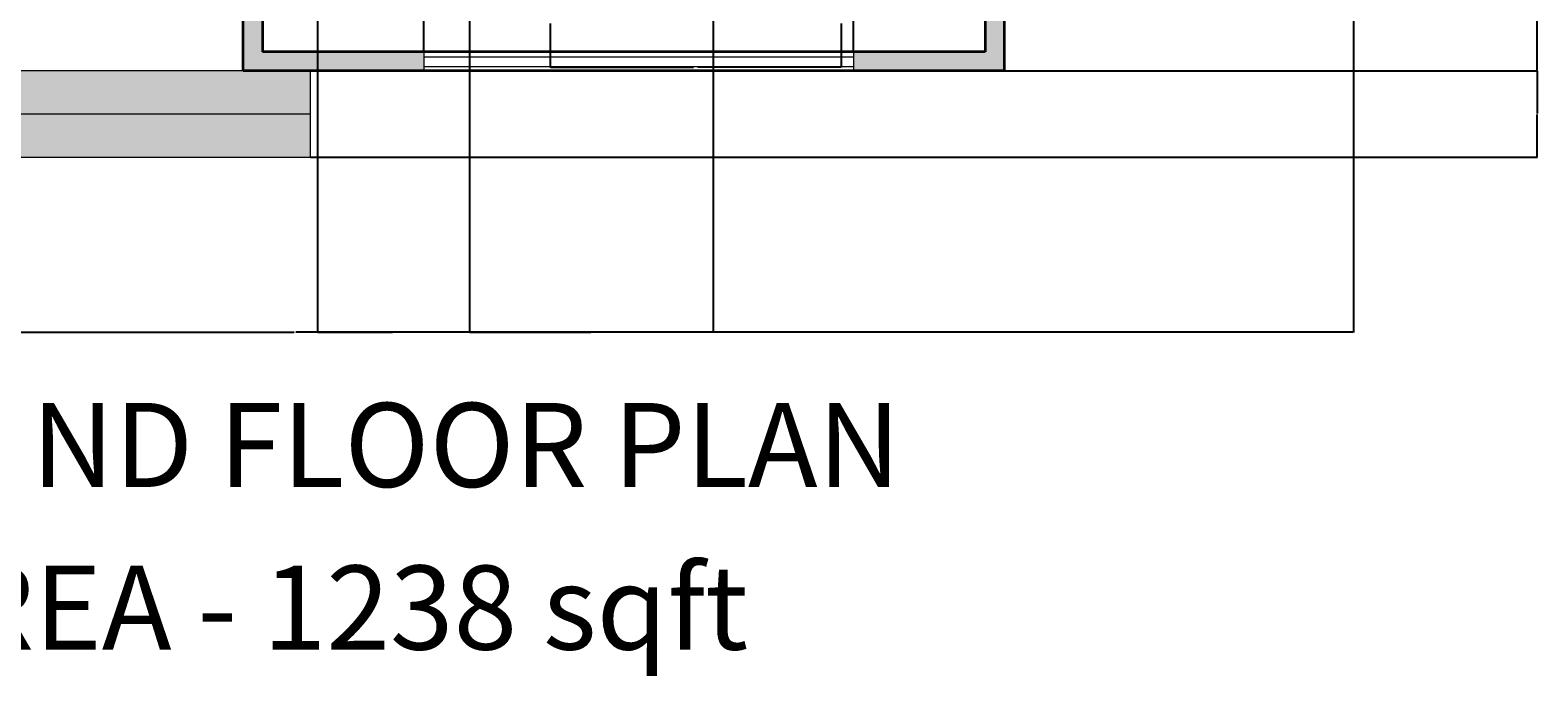
# Model space of a CAD drawing. Units: inches. Extents: x 192 to 1361, y -1362 to 367.
# Tile 10 of 23: x 649 to 1361, y -1362 to -1057. Entities that reach past the tile are written whole.
import ezdxf

# ---------------------------------------------------------------- set-up
doc = ezdxf.new("R2010")
doc.units = ezdxf.units.IN
doc.header["$MEASUREMENT"] = 0
for name, color, linetype, lineweight in [('A-ANNO-DIMS', 2, 'Continuous', 18), ('A-ANNO-TITL', 7, 'Continuous', 35), ('A-FLOR', 8, 'Continuous', 18), ('A-FLOR-STRS', 7, 'Continuous', 18), ('A-WALL-PATT', 250, 'Continuous', 13), ('walls', 7, 'Continuous', 35), ('windows', 4, 'Continuous', 18)]:
    doc.layers.add(name, color=color, linetype=linetype, lineweight=lineweight)
doc.layers.add('A-FLOR-STRS-PATT', color=252, linetype='Continuous', lineweight=13, true_color=0x939598)
doc.styles.get("Standard").update_dxf_attribs({"font": 'arial.ttf'})
doc.dimstyles.get("Standard").update_dxf_attribs({"dimtxt": 0.18, "dimasz": 0.18, "dimexe": 0.18, "dimexo": 0.0625, "dimgap": 0.09, "dimtad": 0, "dimtih": 1, "dimtoh": 1, "dimzin": 0, "dimdsep": 46, "dimlunit": 3, "dimtxsty": 'Standard', "dimcen": 0.09, "dimadec": 0, "dimazin": 0, "dimtfac": 1, "dimtofl": 0, "dimtmove": 0, "dimatfit": 3, "dimfxl": 1, "dimtolj": 1, "dimtzin": 0, "dimarcsym": 0})

# ---------------------------------------------------------------- blocks, each defined once
blk = doc.blocks.new('*D27')
at = {"layer": 'A-ANNO-DIMS', "color": 0, "lineweight": -2, "transparency": 16777216}
for p, q in [((894.63, -1054.34), (894.63, -1075.05)), ((1031.96, -1054.34), (1031.96, -1075.05)), ((894.81, -1074.87), (962.32, -1074.87)), ((1031.78, -1074.87), (964.27, -1074.87))]:
    blk.add_line(p, q, dxfattribs=at)
at = {"layer": 'A-ANNO-DIMS', "color": 0, "transparency": 16777216}
for points in [[(894.81, -1074.84), (894.81, -1074.9), (894.63, -1074.87)], [(1031.78, -1074.84), (1031.78, -1074.9), (1031.96, -1074.87)]]:
    blk.add_solid(points, dxfattribs=at)
at = {"layer": 'Defpoints', "color": 0, "transparency": 16777216}
for p in [(894.63, -1054.27), (1031.96, -1054.27), (1031.96, -1074.87)]:
    blk.add_point(p, dxfattribs=at)
at = {"layer": 'A-ANNO-DIMS', "color": 0, "transparency": 16777216, "insert": (963.29, -1074.87), "char_height": 0.18, "attachment_point": 5}
blk.add_mtext('\\A1;SOFA 137 TYP.', dxfattribs=at)
blk = doc.blocks.new('*D47')
at = {"layer": 'A-ANNO-DIMS', "color": 0, "lineweight": -2, "transparency": 16777216}
for p, q in [((1273.57, -782.95), (1273.57, -1200.05)), ((274.89, -914.5), (274.89, -1200.05)), ((275.07, -1199.87), (773.84, -1199.87)), ((1273.39, -1199.87), (774.62, -1199.87))]:
    blk.add_line(p, q, dxfattribs=at)
at = {"layer": 'A-ANNO-DIMS', "color": 0, "transparency": 16777216}
for points in [[(275.07, -1199.84), (275.07, -1199.9), (274.89, -1199.87)], [(1273.39, -1199.84), (1273.39, -1199.9), (1273.57, -1199.87)]]:
    blk.add_solid(points, dxfattribs=at)
at = {"layer": 'Defpoints', "color": 0, "transparency": 16777216}
for p in [(1273.57, -782.89), (274.89, -914.44), (1273.57, -1199.87)]:
    blk.add_point(p, dxfattribs=at)
at = {"layer": 'A-ANNO-DIMS', "color": 0, "transparency": 16777216, "insert": (774.23, -1199.87), "char_height": 0.18, "attachment_point": 5}
blk.add_mtext('\\A1;998.7', dxfattribs=at)
blk = doc.blocks.new('*D59')
at = {"layer": 'A-ANNO-DIMS', "color": 0, "lineweight": -2, "transparency": 16777216}
for p, q in [((1273.63, -782.89), (1360.41, -782.89)), ((1360.23, -783.07), (1360.23, -929.58)), ((1360.23, -1076.44), (1360.23, -929.94)), ((1108.9, -1076.62), (1360.41, -1076.62))]:
    blk.add_line(p, q, dxfattribs=at)
at = {"layer": 'A-ANNO-DIMS', "color": 0, "transparency": 16777216}
for points in [[(1360.2, -783.07), (1360.26, -783.07), (1360.23, -782.89)], [(1360.2, -1076.44), (1360.26, -1076.44), (1360.23, -1076.62)]]:
    blk.add_solid(points, dxfattribs=at)
at = {"layer": 'Defpoints', "color": 0, "transparency": 16777216}
for p in [(1273.57, -782.89), (1360.23, -782.89), (1108.84, -1076.62)]:
    blk.add_point(p, dxfattribs=at)
at = {"layer": 'A-ANNO-DIMS', "color": 0, "transparency": 16777216, "insert": (1360.23, -929.76), "char_height": 0.18, "attachment_point": 5}
blk.add_mtext('\\A1;293.73', dxfattribs=at)
blk = doc.blocks.new('*D60')
at = {"layer": 'A-ANNO-DIMS', "color": 0, "lineweight": -2, "transparency": 16777216}
for p, q in [((1108.9, -1076.62), (1360.41, -1076.62)), ((1360.23, -1076.8), (1360.23, -1096.79)), ((1360.23, -1117.14), (1360.23, -1097.16)), ((781.62, -1117.32), (1360.41, -1117.32))]:
    blk.add_line(p, q, dxfattribs=at)
at = {"layer": 'A-ANNO-DIMS', "color": 0, "transparency": 16777216}
for points in [[(1360.2, -1076.8), (1360.26, -1076.8), (1360.23, -1076.62)], [(1360.2, -1117.14), (1360.26, -1117.14), (1360.23, -1117.32)]]:
    blk.add_solid(points, dxfattribs=at)
at = {"layer": 'Defpoints', "color": 0, "transparency": 16777216}
for p in [(1108.84, -1076.62), (781.55, -1117.32), (1360.23, -1117.32)]:
    blk.add_point(p, dxfattribs=at)
at = {"layer": 'A-ANNO-DIMS', "color": 0, "transparency": 16777216, "insert": (1360.23, -1096.97), "char_height": 0.18, "attachment_point": 5}
blk.add_mtext('\\A1;40.7', dxfattribs=at)
blk = doc.blocks.new('*D67')
at = {"layer": 'A-ANNO-DIMS', "color": 0, "lineweight": -2, "transparency": 16777216}
for p, q in [((784.8, -597.56), (784.8, -1200.05)), ((856.57, -597.56), (856.57, -1200.05)), ((784.98, -1199.87), (820.29, -1199.87)), ((856.39, -1199.87), (821.08, -1199.87))]:
    blk.add_line(p, q, dxfattribs=at)
at = {"layer": 'A-ANNO-DIMS', "color": 0, "transparency": 16777216}
for points in [[(784.98, -1199.84), (784.98, -1199.9), (784.8, -1199.87)], [(856.39, -1199.84), (856.39, -1199.9), (856.57, -1199.87)]]:
    blk.add_solid(points, dxfattribs=at)
at = {"layer": 'Defpoints', "color": 0, "transparency": 16777216}
for p in [(784.8, -597.5), (856.57, -597.5), (856.57, -1199.87)]:
    blk.add_point(p, dxfattribs=at)
at = {"layer": 'A-ANNO-DIMS', "color": 0, "transparency": 16777216, "insert": (820.69, -1199.87), "char_height": 0.18, "attachment_point": 5}
blk.add_mtext('\\A1;71.76', dxfattribs=at)
blk = doc.blocks.new('*D68')
at = {"layer": 'A-ANNO-DIMS', "color": 0, "lineweight": -2, "transparency": 16777216}
for p, q in [((856.57, -597.56), (856.57, -1200.05)), ((971.58, -597.56), (971.58, -1200.05)), ((856.75, -1199.87), (913.79, -1199.87)), ((971.4, -1199.87), (914.36, -1199.87))]:
    blk.add_line(p, q, dxfattribs=at)
at = {"layer": 'A-ANNO-DIMS', "color": 0, "transparency": 16777216}
for points in [[(856.75, -1199.84), (856.75, -1199.9), (856.57, -1199.87)], [(971.4, -1199.84), (971.4, -1199.9), (971.58, -1199.87)]]:
    blk.add_solid(points, dxfattribs=at)
at = {"layer": 'Defpoints', "color": 0, "transparency": 16777216}
for p in [(856.57, -597.5), (971.58, -597.5), (971.58, -1199.87)]:
    blk.add_point(p, dxfattribs=at)
at = {"layer": 'A-ANNO-DIMS', "color": 0, "transparency": 16777216, "insert": (914.07, -1199.87), "char_height": 0.18, "attachment_point": 5}
blk.add_mtext('\\A1;115', dxfattribs=at)
blk = doc.blocks.new('*D72')
at = {"layer": 'A-ANNO-DIMS', "color": 0, "lineweight": -2, "transparency": 16777216}
for p, q in [((835.08, -1067.56), (835.08, 367.39)), ((835.26, 367.21), (935.95, 367.21)), ((1037.58, 367.21), (936.88, 367.21)), ((1037.76, -1067.56), (1037.76, 367.39))]:
    blk.add_line(p, q, dxfattribs=at)
at = {"layer": 'A-ANNO-DIMS', "color": 0, "transparency": 16777216}
for points in [[(835.26, 367.24), (835.26, 367.18), (835.08, 367.21)], [(1037.58, 367.24), (1037.58, 367.18), (1037.76, 367.21)]]:
    blk.add_solid(points, dxfattribs=at)
at = {"layer": 'Defpoints', "color": 0, "transparency": 16777216}
for p in [(1037.76, 367.21), (835.08, -1067.62), (1037.76, -1067.62)]:
    blk.add_point(p, dxfattribs=at)
at = {"layer": 'A-ANNO-DIMS', "color": 0, "transparency": 16777216, "insert": (936.42, 367.21), "char_height": 0.18, "attachment_point": 5}
blk.add_mtext('\\A1;202.68', dxfattribs=at)

msp = doc.modelspace()

# ---------------------------------------------------------------- hatches: boundary and pattern name
at = {"layer": 'A-FLOR-STRS-PATT'}
h = msp.add_hatch(color=256, dxfattribs=at)
h.dxf.hatch_style = 1
h.paths.add_polyline_path([(781.5537, -1096.9736), (395.2768, -1096.9736), (395.2768, -1117.3227), (781.5537, -1117.3227)])
h.paths.add_polyline_path([(781.5537, -1076.6246), (749.8458, -1076.6246), (441.307, -1076.6246), (395.2768, -1076.6246), (395.2768, -1096.9736), (781.5537, -1096.9736)])
at = {"layer": 'A-WALL-PATT'}
h = msp.add_hatch(color=256, dxfattribs=at)
h.dxf.hatch_style = 1
h.paths.add_polyline_path([(309.5452, 191.102), (300.5452, 191.102), (300.5452, -126.898), (309.5452, -126.898), (309.5452, -117.898)])
h.paths.add_polyline_path([(420.798, 191.102), (337.3229, 191.102), (337.3229, 182.102), (420.798, 182.102)])
h.paths.add_polyline_path([(518.5452, 182.102), (625.4022, 182.102), (625.4022, 191.102), (509.5452, 191.102), (509.5452, 114.3262), (518.5452, 114.3262)])
h.paths.add_polyline_path([(842.5452, 191.102), (763.4438, 191.102), (763.4438, 182.102), (833.5452, 182.102), (833.5452, 161.1615), (836.8088, 161.1615), (842.5452, 161.1615)])
h.paths.add_polyline_path([(842.5452, -16.5675), (833.5452, -16.5675), (833.5452, -60.4996), (784.8041, -60.4996), (784.8041, -354.6796), (793.8041, -354.6796), (793.8041, -69.4996), (1094.1252, -69.4996), (1094.1252, -60.4996), (842.5452, -60.4996)])
h.paths.add_polyline_path([(518.5452, 36.602), (509.5452, 36.602), (509.5452, -117.898), (420.2204, -117.898), (420.2204, -126.898), (518.5452, -126.898)])
h.paths.add_polyline_path([(474.8041, -377.0384), (465.8041, -377.0384), (465.8041, -381.5384), (465.8041, -450.898), (537.5717, -450.898), (537.5717, -441.898), (474.8041, -441.898)])
h.paths.add_polyline_path([(1162.8041, -380.6763), (1204.3001, -380.6763), (1204.3001, -375.6763), (1195.1471, -375.6763), (1153.8041, -375.6763), (1153.8041, -448.4996), (856.5691, -448.4996), (856.5691, -457.4996), (1162.8041, -457.4996)])
h.paths.add_polyline_path([(1162.8041, -525.128), (1153.8041, -525.128), (1153.8041, -597.4996), (1162.8041, -597.4996)], flags=17)
h.paths.add_polyline_path([(1162.8041, -60.4996), (1153.8041, -60.4996), (1153.8041, -69.4996), (1153.8041, -177.4733), (1205.8889, -177.4733), (1205.8889, -172.4733), (1162.8041, -172.4733)])
h.paths.add_polyline_path([(980.5799, -525.686), (971.5799, -525.686), (971.5799, -597.4996), (980.5799, -597.4996)], flags=17)
h.paths.add_polyline_path([(856.5691, -448.4996), (798.7542, -448.4996), (784.8041, -448.4996), (784.8041, -457.4996), (847.5691, -457.4996), (847.5691, -597.4996), (784.8041, -597.4996), (784.8041, -606.4996), (1273.5658, -606.4996), (1273.5658, -597.4996), (856.5691, -597.4996)])
h.paths.add_polyline_path([(1273.5658, -773.892), (1099.8366, -773.892), (1099.8366, -851.9362), (1108.8366, -851.9362), (1108.8366, -782.892), (1273.5658, -782.892)])
h.paths.add_polyline_path([(1108.8366, -982.9214), (1099.8366, -982.9214), (1099.8366, -1067.6246), (1037.7563, -1067.6246), (1037.7563, -1076.6246), (1108.8366, -1076.6246)])
h.paths.add_polyline_path([(835.078, -1067.6246), (758.8458, -1067.6246), (758.8458, -940.2324), (749.8458, -940.2324), (749.8458, -963.172), (749.8458, -970.4644), (749.8458, -1076.6246), (835.078, -1076.6246)])
h.paths.add_polyline_path([(450.307, -1066.9838), (441.307, -1066.9838), (441.307, -1076.6246), (450.307, -1076.6246)])
h.paths.add_polyline_path([(492.8925, -756.4415), (274.8925, -756.4415), (274.8925, -765.4415), (492.8925, -765.4415)])
h.paths.add_polyline_path([(283.8925, -835.2244), (274.8925, -835.2244), (274.8925, -914.4415), (492.8925, -914.4415), (492.8925, -839.9415), (483.8925, -839.9415), (483.8925, -905.4415), (283.8925, -905.4415)])
h.paths.add_polyline_path([(283.8925, -441.898), (283.8925, -375.4296), (281.6021, -375.4296), (281.6021, -399.4121), (274.8925, -399.4121), (274.8925, -441.898), (274.8925, -684.5089), (283.8925, -684.5089)])

# ---------------------------------------------------------------- linework, layer by layer
at = {"layer": 'A-FLOR'}
msp.add_line((749.8458, -1076.6246), (441.307, -1076.6246), dxfattribs=at)
at = {"layer": 'A-FLOR-STRS'}
for p, q in [((781.5537, -1117.3227), (781.5537, -1076.6246)), ((395.2768, -1096.9736), (781.5537, -1096.9736)), ((395.2768, -1117.3227), (781.5537, -1117.3227))]:
    msp.add_line(p, q, dxfattribs=at)
at = {"layer": 'walls'}
for p, q in [((1099.8366, -773.892), (1099.8366, -1067.6246)), ((1108.8366, -782.892), (1108.8366, -1076.6246)), ((749.8458, -1076.6246), (749.8458, -940.2324)), ((758.8458, -940.2324), (758.8458, -1067.6246)), ((1099.8366, -1067.6246), (758.8458, -1067.6246)), ((1108.8366, -1076.6246), (749.8458, -1076.6246))]:
    msp.add_line(p, q, dxfattribs=at)
at = {"layer": 'windows'}
for p, q in [((835.078, -1067.6246), (835.078, -1076.6246)), ((835.078, -1070.0396), (1037.7563, -1070.0396)), ((1037.7563, -1067.6246), (1037.7563, -1076.6246)), ((835.078, -1074.6014), (1037.7563, -1074.6014))]:
    msp.add_line(p, q, dxfattribs=at)

# ---------------------------------------------------------------- texts
at = {"layer": 'A-ANNO-TITL'}
for s, p in [('GROUND FLOOR PLAN', (499.1662, -1272.9554)), ('AREA - 1238 sqft', (584.0247, -1349.6751))]:
    msp.add_text(s, height=39.646878, dxfattribs=at).set_placement(p)

# ---------------------------------------------------------------- dimensions: what is measured, and where the dimension line sits
at = {"layer": 'A-ANNO-DIMS'}
for base, p1, p2, override, picture, middle in [((1037.7563, 367.2097), (835.078, -1067.6246), (1037.7563, -1067.6246), {"dimdec": 2, "dimlfac": 1, "dimrnd": 0, "dimzin": 0, "dimdsep": 46, "dimlunit": 2}, '*D72', (936.4171, 367.2097)), ((856.56907, -1199.87271), (784.80414, -597.49959), (856.56907, -597.49959), {"dimdec": 2, "dimlfac": 1, "dimrnd": 0, "dimzin": 0, "dimdsep": 46, "dimlunit": 2}, '*D67', (820.68661, -1199.87271)), ((971.5799, -1199.8727), (856.5691, -597.4996), (971.5799, -597.4996), {"dimdec": 0, "dimlfac": 1, "dimrnd": 0, "dimzin": 0, "dimdsep": 46, "dimlunit": 2}, '*D68', (914.0745, -1199.8727)), ((1273.5658, -1199.8727), (274.8925, -914.4415), (1273.5658, -782.892), {"dimdec": 1, "dimlfac": 1, "dimrnd": 0, "dimzin": 0, "dimdsep": 46, "dimlunit": 2}, '*D47', (774.2292, -1199.8727))]:
    dim = msp.add_linear_dim(base=base, p1=p1, p2=p2, dimstyle='Standard', override=override, dxfattribs=at)
    dim.commit()
    dim.dimension.update_dxf_attribs({"geometry": picture, "text_midpoint": middle})
for base, p2, override, picture, middle in [((1360.2331, -782.892), (1273.5658, -782.892), {"dimdec": 2, "dimlfac": 1, "dimrnd": 0, "dimzin": 0, "dimdsep": 46, "dimlunit": 2}, '*D59', (1360.2331, -929.7583)), ((1360.2331, -1117.3227), (781.5537, -1117.3227), {"dimdec": 1, "dimlfac": 1, "dimrnd": 0, "dimzin": 0, "dimdsep": 46, "dimlunit": 2}, '*D60', (1360.2331, -1096.9736))]:
    dim = msp.add_linear_dim(base=base, p1=(1108.8366, -1076.6246), p2=p2, angle=90, dimstyle='Standard', override=override, dxfattribs=at)
    dim.commit()
    dim.dimension.update_dxf_attribs({"geometry": picture, "text_midpoint": middle})
dim = msp.add_linear_dim(base=(1031.9563, -1074.8726), p1=(894.6259, -1054.273), p2=(1031.9563, -1054.273), text='SOFA <> TYP.', dimstyle='Standard', override={"dimdec": 0, "dimlfac": 1, "dimrnd": 0, "dimzin": 0, "dimdsep": 46, "dimlunit": 2}, dxfattribs=at)
dim.commit()
dim.dimension.update_dxf_attribs({"geometry": '*D27', "text_midpoint": (963.2911, -1074.8726)})

doc.saveas('drawing.dxf')
